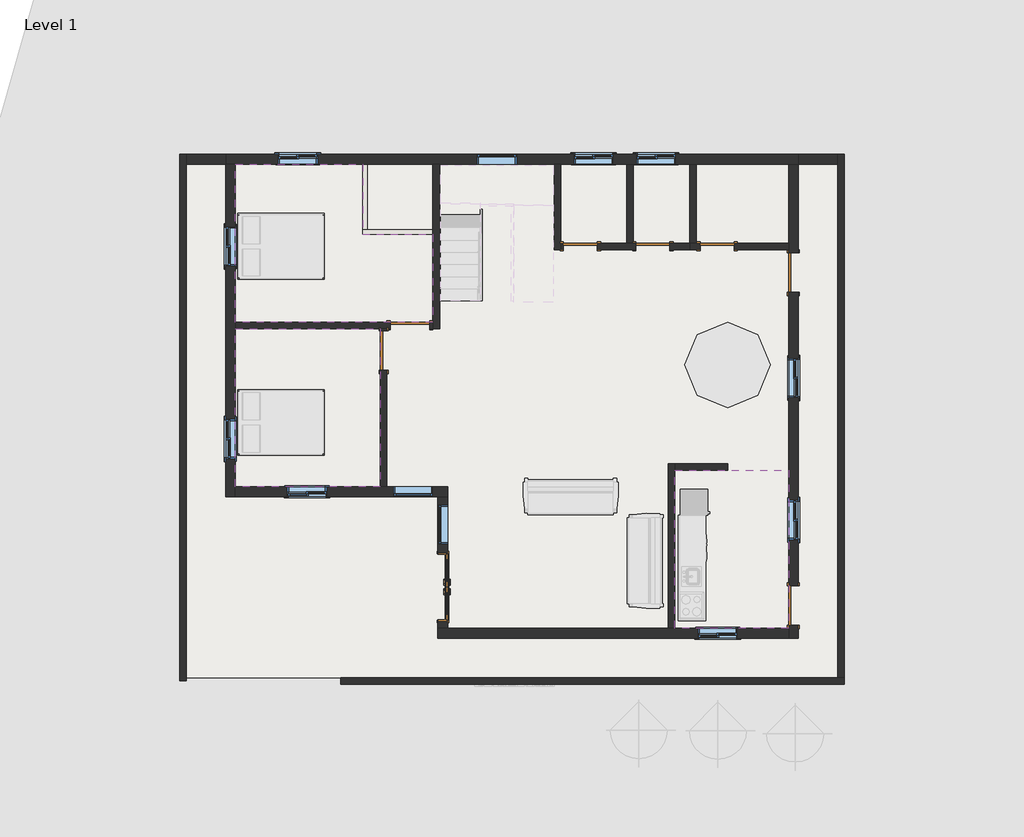
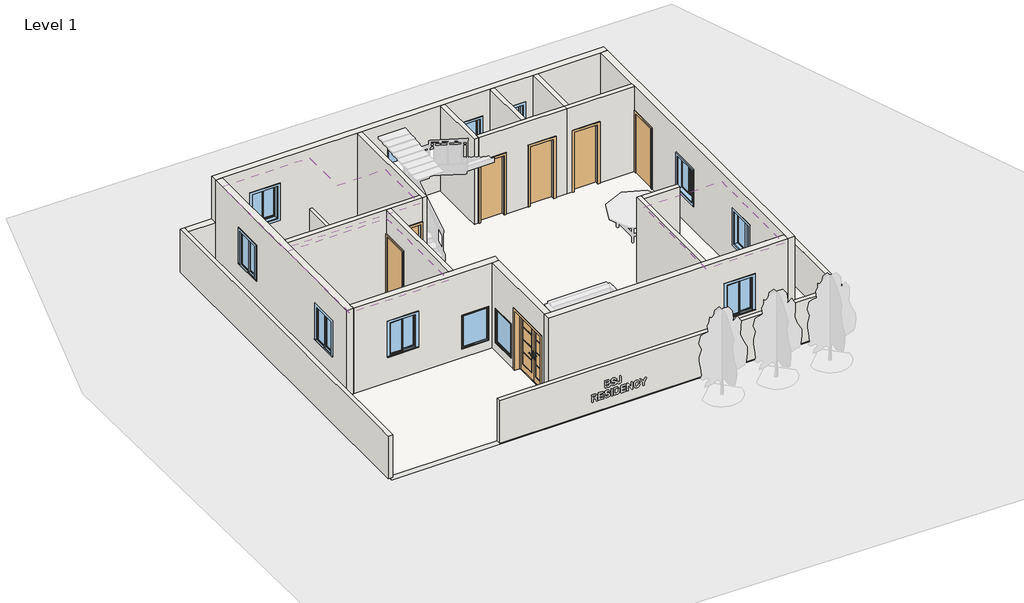
# One storey, part 1 of 2: 23 walls, 12 windows, 8 doors, 3 coverings, 1 slab.
"""IFC4 building model written with IfcOpenShell, lengths in millimetres."""

from ifc_helpers import new_model, si_unit, frame, origin, origin_with_axes, place, context, project, spatial, polyline, outline, extrude, faceted_brep, transform, mapped, element, save
from components import door_014e9f54, door_dc34e247, door_16372e1c, door_a90ba1ad, door_0ca8825f, window_c1f32544, window_26734613, window_e25db5b6

model = new_model("IFC4")

# Units and contexts
model_context = context("Model", 3, world=origin())
ifc_project = project(units=[si_unit("LENGTHUNIT", "METRE", prefix="MILLI")], contexts=[model_context])

# Site, building, storey
site = spatial("IfcSite", under=ifc_project)
building = spatial("IfcBuilding", under=site)
storey = spatial("IfcBuildingStorey", under=building, Name="Level 1", Elevation=0.0)

# Coverings
placement = place(None, origin())
element("IfcCovering", 1, ObjectType="2' x 4' ACT System", at=placement, inside=storey, context=model_context, shape_type="SweptSolid", body=[
    extrude(outline(polyline([(-8845.5867944, 6769.3230289), (-12198.3867944, 6769.3230289), (-12198.3867944, 10426.9230289), (-8845.5867944, 10426.9230289), (-8845.5867944, 6769.3230289)])), frame((0.0, 0.0, 2743.2), z_axis=(0.0, 0.0, 1.0), x_axis=(1.0, 0.0, 0.0)), (0.0, 0.0, 1.0), 57.15),
])
element("IfcCovering", 2, ObjectType="2' x 4' ACT System", at=placement, inside=storey, context=model_context, shape_type="SweptSolid", body=[
    extrude(outline(polyline([(-12198.3867944, 10579.3230289), (-12198.3867944, 14236.9230289), (-9251.9867944, 14236.9230289), (-9251.9867944, 12611.3230289), (-7626.3867944, 12611.3230289), (-7626.3867944, 10579.3230289), (-12198.3867944, 10579.3230289)])), frame((0.0, 0.0, 2743.2), z_axis=(0.0, 0.0, 1.0), x_axis=(1.0, 0.0, 0.0)), (0.0, 0.0, 1.0), 57.15),
])
element("IfcCovering", 3, ObjectType="2' x 4' ACT System", at=placement, inside=storey, context=model_context, shape_type="SweptSolid", body=[
    extrude(outline(polyline([(603.2132056, 7150.3230289), (603.2132056, 3492.7230289), (-2025.6867944, 3492.7230289), (-2025.6867944, 7150.3230289), (603.2132056, 7150.3230289)])), frame((0.0, 0.0, 2743.2), z_axis=(0.0, 0.0, 1.0), x_axis=(1.0, 0.0, 0.0)), (0.0, 0.0, 1.0), 57.15),
])

# Doors
door_shape = door_014e9f54(model_context)
element("IfcDoor", 4, ObjectType="Door-Exterior-Double-Full Glass-Wood_Clad : 60\" x 84\"", at=placement, inside=storey, context=model_context, shape_type="MappedRepresentation", body=[
    mapped(door_shape, transform((-7394.6117944, 4445.2230289, 0.0), x_axis=(0.0, -1.0, 0.0), y_axis=(1.0, 0.0, 0.0), z_axis=(0.0, 0.0, 1.0))),
])
door_2_shape = door_dc34e247(model_context)
element("IfcDoor", 5, ObjectType="Single-Flush : 2'7\"", at=placement, inside=storey, context=model_context, shape_type="MappedRepresentation", body=[
    mapped(door_2_shape, transform((-4212.7737939, 12331.9230289, 0.0), x_axis=(-1.0, 0.0, 0.0), y_axis=(0.0, -1.0, 0.0), z_axis=(0.0, 0.0, 1.0))),
])
element("IfcDoor", 6, ObjectType="Single-Flush : 2'7\"", at=placement, inside=storey, context=model_context, shape_type="MappedRepresentation", body=[
    mapped(door_2_shape, transform((-2536.3737939, 12331.9230289, 0.0), x_axis=(-1.0, 0.0, 0.0), y_axis=(0.0, -1.0, 0.0), z_axis=(0.0, 0.0, 1.0))),
])
element("IfcDoor", 7, ObjectType="Single-Flush : 2'7\"", at=placement, inside=storey, context=model_context, shape_type="MappedRepresentation", body=[
    mapped(door_2_shape, transform((-1047.7867944, 12331.9230289, 0.0), x_axis=(-1.0, 0.0, 0.0), y_axis=(0.0, -1.0, 0.0), z_axis=(0.0, 0.0, 1.0))),
])
door_3_shape = door_16372e1c(model_context)
element("IfcDoor", 8, ObjectType="Single-Flush : 36\" x 84\"", at=placement, inside=storey, context=model_context, shape_type="MappedRepresentation", body=[
    mapped(door_3_shape, transform((-8159.7867944, 10503.1230289, 0.0), x_axis=(1.0, 0.0, 0.0), y_axis=(0.0, 1.0, 0.0), z_axis=(0.0, 0.0, 1.0))),
])
element("IfcDoor", 9, ObjectType="Single-Flush : 36\" x 84\"", at=placement, inside=storey, context=model_context, shape_type="MappedRepresentation", body=[
    mapped(door_3_shape, transform((-8769.3867944, 9918.9230289, 0.0), x_axis=(0.0, 1.0, 0.0), y_axis=(-1.0, 0.0, 0.0), z_axis=(0.0, 0.0, 1.0))),
])
door_4_shape = door_a90ba1ad(model_context)
element("IfcDoor", 10, ObjectType="Single-Flush : 36\" x 84\"", at=placement, inside=storey, context=model_context, shape_type="MappedRepresentation", body=[
    mapped(door_4_shape, transform((717.5132056, 4013.4230289, 0.0), x_axis=(0.0, -1.0, 0.0), y_axis=(1.0, 0.0, 0.0), z_axis=(0.0, 0.0, 1.0))),
])
door_5_shape = door_0ca8825f(model_context)
element("IfcDoor", 11, ObjectType="Single-Flush : 36\" x 84\"", at=placement, inside=storey, context=model_context, shape_type="MappedRepresentation", body=[
    mapped(door_5_shape, transform((717.5132056, 11722.3230289, 0.0), x_axis=(0.0, 1.0, 0.0), y_axis=(-1.0, 0.0, 0.0), z_axis=(0.0, 0.0, 1.0))),
])

# Slab
element("IfcSlab", 12, ObjectType="6\"", at=placement, inside=storey, context=model_context, shape_type="SweptSolid", body=[
    extrude(outline(polyline([(1746.2132056, 14236.9230289), (1746.2132056, 2349.7230289), (-13341.3867944, 2349.7230289), (-13341.3867944, 14236.9230289), (1746.2132056, 14236.9230289)])), frame((0.0, 0.0, -152.4), z_axis=(0.0, 0.0, 1.0), x_axis=(1.0, 0.0, 0.0)), (0.0, 0.0, 1.0), 152.4),
])

# Walls
element("IfcWall", 13, ObjectType="4\"", at=placement, inside=storey, context=model_context, shape_type="Brep", body=[
    faceted_brep([(-7626.3867944, 12712.9230289, 0.0), (-9150.3867944, 12712.9230289, 0.0), (-9251.9867944, 12712.9230289, 0.0), (-9251.9867944, 12712.9230289, 914.4), (-9150.3867944, 12712.9230289, 914.4), (-7626.3867944, 12712.9230289, 914.4), (-7626.3867944, 12611.3230289, 0.0), (-7626.3867944, 12611.3230289, 914.4), (-9251.9867944, 12611.3230289, 914.4), (-9251.9867944, 12611.3230289, 0.0)], [[[0, 1, 2, 3, 4, 5]], [[6, 7, 8, 9]], [[2, 1, 0, 6, 9]], [[5, 4, 3, 8, 7]], [[0, 5, 7, 6]], [[3, 2, 9, 8]]]),
])
element("IfcWall", 14, ObjectType="4\"", at=placement, inside=storey, context=model_context, shape_type="SweptSolid", body=[
    extrude(outline(polyline([(-9150.3867944, 14236.9230289), (-9150.3867944, 12712.9230289), (-9251.9867944, 12712.9230289), (-9251.9867944, 14236.9230289), (-9150.3867944, 14236.9230289)])), origin_with_axes(), (0.0, 0.0, 1.0), 914.4),
])
element("IfcWall", 15, ObjectType="6\"", at=placement, inside=storey, context=model_context, shape_type="Brep", body=[
    faceted_brep([(-13341.3867944, 2273.5230289, 0.0), (-13341.3867944, 14236.9230289, 0.0), (-13341.3867944, 14465.5230289, 0.0), (-13341.3867944, 14465.5230289, 1524.0), (-13341.3867944, 14236.9230289, 1524.0), (-13341.3867944, 2273.5230289, 1524.0), (-13493.7867944, 2273.5230289, 0.0), (-13493.7867944, 2273.5230289, 1524.0), (-13493.7867944, 14465.5230289, 1524.0), (-13493.7867944, 14465.5230289, 0.0)], [[[0, 1, 2, 3, 4, 5]], [[6, 7, 8, 9]], [[2, 1, 0, 6, 9]], [[5, 4, 3, 8, 7]], [[0, 5, 7, 6]], [[3, 2, 9, 8]]]),
])
element("IfcWall", 16, ObjectType="6\"", at=placement, inside=storey, context=model_context, shape_type="Brep", body=[
    faceted_brep([(1898.6132056, 2349.7230289, 0.0), (1746.2132056, 2349.7230289, 0.0), (-9759.9867944, 2349.7230289, 0.0), (-9759.9867944, 2349.7230289, 1524.0), (1746.2132056, 2349.7230289, 1524.0), (1898.6132056, 2349.7230289, 1524.0), (1898.6132056, 2197.3230289, 0.0), (1898.6132056, 2197.3230289, 1524.0), (-9759.9867944, 2197.3230289, 1524.0), (-9759.9867944, 2197.3230289, 0.0)], [[[0, 1, 2, 3, 4, 5]], [[6, 7, 8, 9]], [[2, 1, 0, 6, 9]], [[3, 2, 9, 8]], [[5, 4, 3, 8, 7]], [[0, 5, 7, 6]]]),
])
element("IfcWall", 17, ObjectType="6\"", at=placement, inside=storey, context=model_context, shape_type="Brep", body=[
    faceted_brep([(1746.2132056, 14465.5230289, 0.0), (1746.2132056, 14236.9230289, 0.0), (1746.2132056, 2349.7230289, 0.0), (1746.2132056, 2349.7230289, 1524.0), (1746.2132056, 14236.9230289, 1524.0), (1746.2132056, 14465.5230289, 1524.0), (1898.6132056, 14465.5230289, 0.0), (1898.6132056, 14465.5230289, 1524.0), (1898.6132056, 2349.7230289, 1524.0), (1898.6132056, 2349.7230289, 0.0)], [[[0, 1, 2, 3, 4, 5]], [[6, 7, 8, 9]], [[2, 1, 0, 6, 9]], [[5, 4, 3, 8, 7]], [[3, 2, 9, 8]], [[0, 5, 7, 6]]]),
])
element("IfcWall", 18, ObjectType="6\"", at=placement, inside=storey, context=model_context, shape_type="Brep", body=[
    faceted_brep([(-7626.3867944, 14236.9230289, 0.0), (-7626.3867944, 12712.9230289, 0.0), (-7626.3867944, 12611.3230289, 0.0), (-7626.3867944, 10579.3230289, 0.0), (-7626.3867944, 10426.9230289, 0.0), (-7626.3867944, 10426.9230289, 3048.0), (-7626.3867944, 10579.3230289, 3048.0), (-7626.3867944, 14236.9230289, 3048.0), (-7473.9867944, 14236.9230289, 0.0), (-7473.9867944, 14236.9230289, 3048.0), (-7473.9867944, 10426.9230289, 3048.0), (-7473.9867944, 10426.9230289, 0.0)], [[[0, 1, 2, 3, 4, 5, 6, 7]], [[8, 9, 10, 11]], [[4, 3, 2, 1, 0, 8, 11]], [[7, 6, 5, 10, 9]], [[0, 7, 9, 8]], [[5, 4, 11, 10]]]),
])
element("IfcWall", 19, ObjectType="6\"", at=placement, inside=storey, context=model_context, shape_type="Brep", body=[
    faceted_brep([(-7626.3867944, 10579.3230289, 0.0), (-7702.5867944, 10579.3230289, 0.0), (-7702.5867944, 10579.3230289, 2133.6), (-8616.9867944, 10579.3230289, 2133.6), (-8616.9867944, 10579.3230289, 0.0), (-12198.3867944, 10579.3230289, 0.0), (-12198.3867944, 10579.3230289, 3048.0), (-7626.3867944, 10579.3230289, 3048.0), (-7702.5867944, 10426.9230289, 2133.6), (-7702.5867944, 10426.9230289, 0.0), (-7626.3867944, 10426.9230289, 0.0), (-7626.3867944, 10426.9230289, 3048.0), (-8693.1867944, 10426.9230289, 3048.0), (-8845.5867944, 10426.9230289, 3048.0), (-12198.3867944, 10426.9230289, 3048.0), (-12198.3867944, 10426.9230289, 0.0), (-8845.5867944, 10426.9230289, 0.0), (-8693.1867944, 10426.9230289, 0.0), (-8616.9867944, 10426.9230289, 0.0), (-8616.9867944, 10426.9230289, 2133.6)], [[[0, 1, 2, 3, 4, 5, 6, 7]], [[8, 9, 10, 11, 12, 13, 14, 15, 16, 17, 18, 19]], [[10, 9, 1, 0]], [[18, 17, 16, 15, 5, 4]], [[7, 6, 14, 13, 12, 11]], [[0, 7, 11, 10]], [[6, 5, 15, 14]], [[2, 1, 9, 8]], [[3, 2, 8, 19]], [[4, 3, 19, 18]]]),
])
element("IfcWall", 20, ObjectType="6\"", at=placement, inside=storey, context=model_context, shape_type="SweptSolid", body=[
    extrude(outline(polyline([(10426.9230289, 0.0), (10376.1230289, 0.0), (10376.1230289, 2133.6), (9461.7230289, 2133.6), (9461.7230289, 0.0), (6769.3230289, 0.0), (6769.3230289, 3048.0), (10426.9230289, 3048.0), (10426.9230289, 0.0)])), frame((-8845.5867944, 0.0, 0.0), z_axis=(1.0, 0.0, 0.0), x_axis=(0.0, 1.0, 0.0)), (0.0, 0.0, 1.0), 152.4),
])
element("IfcWall", 21, ObjectType="6\"", at=placement, inside=storey, context=model_context, shape_type="Brep", body=[
    faceted_brep([(-1441.4867944, 12408.1230289, 2133.6), (-1441.4867944, 12408.1230289, 0.0), (-1530.3867944, 12408.1230289, 0.0), (-1682.7867944, 12408.1230289, 0.0), (-1682.7867944, 12408.1230289, 3048.0), (-1530.3867944, 12408.1230289, 3048.0), (603.2132056, 12408.1230289, 3048.0), (603.2132056, 12408.1230289, 0.0), (-654.0867944, 12408.1230289, 0.0), (-654.0867944, 12408.1230289, 2133.6), (-1682.7867944, 12255.7230289, 0.0), (-1441.4867944, 12255.7230289, 0.0), (-1441.4867944, 12255.7230289, 2133.6), (-654.0867944, 12255.7230289, 2133.6), (-654.0867944, 12255.7230289, 0.0), (603.2132056, 12255.7230289, 0.0), (603.2132056, 12255.7230289, 3048.0), (-1682.7867944, 12255.7230289, 3048.0)], [[[0, 1, 2, 3, 4, 5, 6, 7, 8, 9]], [[10, 11, 12, 13, 14, 15, 16, 17]], [[8, 7, 15, 14]], [[3, 2, 1, 11, 10]], [[6, 5, 4, 17, 16]], [[7, 6, 16, 15]], [[4, 3, 10, 17]], [[12, 11, 1, 0]], [[13, 12, 0, 9]], [[14, 13, 9, 8]]]),
])
element("IfcWall", 22, ObjectType="6\"", at=placement, inside=storey, context=model_context, shape_type="SweptSolid", body=[
    extrude(outline(polyline([(-1530.3867944, 14236.9230289), (-1530.3867944, 12408.1230289), (-1682.7867944, 12408.1230289), (-1682.7867944, 14236.9230289), (-1530.3867944, 14236.9230289)])), origin_with_axes(), (0.0, 0.0, 1.0), 3048.0),
])
element("IfcWall", 23, ObjectType="6\"", at=placement, inside=storey, context=model_context, shape_type="Brep", body=[
    faceted_brep([(-4822.3737939, 14236.9230289, 0.0), (-4822.3737939, 12255.7230289, 0.0), (-4822.3737939, 12255.7230289, 3048.0), (-4822.3737939, 14236.9230289, 3048.0), (-4669.9737939, 14236.9230289, 0.0), (-4669.9737939, 14236.9230289, 3048.0), (-4669.9737939, 12408.1230289, 3048.0), (-4669.9737939, 12255.7230289, 3048.0), (-4669.9737939, 12255.7230289, 0.0), (-4669.9737939, 12408.1230289, 0.0)], [[[0, 1, 2, 3]], [[4, 5, 6, 7, 8, 9]], [[1, 0, 4, 9, 8]], [[3, 2, 7, 6, 5]], [[2, 1, 8, 7]], [[0, 3, 5, 4]]]),
])
element("IfcWall", 24, ObjectType="6\"", at=placement, inside=storey, context=model_context, shape_type="Brep", body=[
    faceted_brep([(-3819.0737939, 12255.7230289, 0.0), (-2930.0737939, 12255.7230289, 0.0), (-2930.0737939, 12255.7230289, 2133.6), (-2142.6737939, 12255.7230289, 2133.6), (-2142.6737939, 12255.7230289, 0.0), (-1682.7867944, 12255.7230289, 0.0), (-1682.7867944, 12255.7230289, 3048.0), (-4669.9737939, 12255.7230289, 3048.0), (-4669.9737939, 12255.7230289, 0.0), (-4606.4737939, 12255.7230289, 0.0), (-4606.4737939, 12255.7230289, 2133.6), (-3819.0737939, 12255.7230289, 2133.6), (-2930.0737939, 12408.1230289, 2133.6), (-2930.0737939, 12408.1230289, 0.0), (-2993.5737939, 12408.1230289, 0.0), (-3145.9737939, 12408.1230289, 0.0), (-3819.0737939, 12408.1230289, 0.0), (-3819.0737939, 12408.1230289, 2133.6), (-4606.4737939, 12408.1230289, 2133.6), (-4606.4737939, 12408.1230289, 0.0), (-4669.9737939, 12408.1230289, 0.0), (-4669.9737939, 12408.1230289, 3048.0), (-3145.9737939, 12408.1230289, 3048.0), (-2993.5737939, 12408.1230289, 3048.0), (-1682.7867944, 12408.1230289, 3048.0), (-1682.7867944, 12408.1230289, 0.0), (-2142.6737939, 12408.1230289, 0.0), (-2142.6737939, 12408.1230289, 2133.6)], [[[0, 1, 2, 3, 4, 5, 6, 7, 8, 9, 10, 11]], [[12, 13, 14, 15, 16, 17, 18, 19, 20, 21, 22, 23, 24, 25, 26, 27]], [[20, 19, 9, 8]], [[26, 25, 5, 4]], [[16, 15, 14, 13, 1, 0]], [[7, 6, 24, 23, 22, 21]], [[8, 7, 21, 20]], [[6, 5, 25, 24]], [[10, 9, 19, 18]], [[11, 10, 18, 17]], [[0, 11, 17, 16]], [[2, 1, 13, 12]], [[3, 2, 12, 27]], [[4, 3, 27, 26]]]),
])
element("IfcWall", 25, ObjectType="6\"", at=placement, inside=storey, context=model_context, shape_type="SweptSolid", body=[
    extrude(outline(polyline([(-2993.5737939, 14236.9230289), (-2993.5737939, 12408.1230289), (-3145.9737939, 12408.1230289), (-3145.9737939, 14236.9230289), (-2993.5737939, 14236.9230289)])), origin_with_axes(), (0.0, 0.0, 1.0), 3048.0),
])
element("IfcWall", 26, ObjectType="6\"", at=placement, inside=storey, context=model_context, shape_type="Brep", body=[
    faceted_brep([(-2025.6867944, 3492.7230289, 0.0), (-2025.6867944, 7150.3230289, 0.0), (-2025.6867944, 7302.7230289, 0.0), (-2025.6867944, 7302.7230289, 3048.0), (-2025.6867944, 7150.3230289, 3048.0), (-2025.6867944, 3492.7230289, 3048.0), (-2178.0867944, 3492.7230289, 0.0), (-2178.0867944, 3492.7230289, 3048.0), (-2178.0867944, 7302.7230289, 3048.0), (-2178.0867944, 7302.7230289, 0.0)], [[[0, 1, 2, 3, 4, 5]], [[6, 7, 8, 9]], [[2, 1, 0, 6, 9]], [[5, 4, 3, 8, 7]], [[0, 5, 7, 6]], [[3, 2, 9, 8]]]),
])
element("IfcWall", 27, ObjectType="6\"", at=placement, inside=storey, context=model_context, shape_type="SweptSolid", body=[
    extrude(outline(polyline([(-806.4867944, 7150.3230289), (-2025.6867944, 7150.3230289), (-2025.6867944, 7302.7230289), (-806.4867944, 7302.7230289), (-806.4867944, 7150.3230289)])), origin_with_axes(), (0.0, 0.0, 1.0), 3048.0),
])
element("IfcWall", 28, ObjectType="9\"", at=placement, inside=storey, context=model_context, shape_type="SweptSolid", body=[
    extrude(outline(polyline([(-12426.9867944, 14236.9230289), (-13341.3867944, 14236.9230289), (-13341.3867944, 14465.5230289), (-12426.9867944, 14465.5230289), (-12426.9867944, 14236.9230289)])), origin_with_axes(), (0.0, 0.0, 1.0), 1524.0),
])
element("IfcWall", 29, ObjectType="9\"", at=placement, inside=storey, context=model_context, shape_type="Brep", body=[
    faceted_brep([(-12426.9867944, 14236.9230289, 3048.0), (-12426.9867944, 14236.9230289, 0.0), (-12426.9867944, 6540.7230289, 0.0), (-12426.9867944, 6540.7230289, 3048.0), (-12426.9867944, 8331.4230289, 2133.6), (-12426.9867944, 7417.0230289, 2133.6), (-12426.9867944, 7417.0230289, 914.4), (-12426.9867944, 8331.4230289, 914.4), (-12426.9867944, 12789.1230289, 2133.6), (-12426.9867944, 11874.7230289, 2133.6), (-12426.9867944, 11874.7230289, 914.4), (-12426.9867944, 12789.1230289, 914.4), (-12198.3867944, 14236.9230289, 0.0), (-12198.3867944, 14236.9230289, 3048.0), (-12198.3867944, 10579.3230289, 3048.0), (-12198.3867944, 10426.9230289, 3048.0), (-12198.3867944, 6769.3230289, 3048.0), (-12198.3867944, 6540.7230289, 3048.0), (-12198.3867944, 6540.7230289, 0.0), (-12198.3867944, 6769.3230289, 0.0), (-12198.3867944, 10426.9230289, 0.0), (-12198.3867944, 10579.3230289, 0.0), (-12198.3867944, 8331.4230289, 2133.6), (-12198.3867944, 8331.4230289, 914.4), (-12198.3867944, 7417.0230289, 914.4), (-12198.3867944, 7417.0230289, 2133.6), (-12198.3867944, 12789.1230289, 2133.6), (-12198.3867944, 12789.1230289, 914.4), (-12198.3867944, 11874.7230289, 914.4), (-12198.3867944, 11874.7230289, 2133.6)], [[[0, 1, 2, 3], [4, 5, 6, 7], [8, 9, 10, 11]], [[12, 13, 14, 15, 16, 17, 18, 19, 20, 21], [22, 23, 24, 25], [26, 27, 28, 29]], [[2, 1, 12, 21, 20, 19, 18]], [[3, 2, 18, 17]], [[0, 3, 17, 16, 15, 14, 13]], [[23, 22, 4, 7]], [[24, 23, 7, 6]], [[25, 24, 6, 5]], [[22, 25, 5, 4]], [[27, 26, 8, 11]], [[28, 27, 11, 10]], [[29, 28, 10, 9]], [[26, 29, 9, 8]], [[0, 13, 12, 1]]]),
])
element("IfcWall", 30, ObjectType="9\"", at=placement, inside=storey, context=model_context, shape_type="Brep", body=[
    faceted_brep([(603.2132056, 14236.9230289, 0.0), (603.2132056, 12408.1230289, 0.0), (603.2132056, 12255.7230289, 0.0), (603.2132056, 12179.5230289, 0.0), (603.2132056, 12179.5230289, 2133.6), (603.2132056, 11265.1230289, 2133.6), (603.2132056, 11265.1230289, 0.0), (603.2132056, 4470.6230289, 0.0), (603.2132056, 4470.6230289, 2133.6), (603.2132056, 3556.2230289, 2133.6), (603.2132056, 3556.2230289, 0.0), (603.2132056, 3492.7230289, 0.0), (603.2132056, 3264.1230289, 0.0), (603.2132056, 3264.1230289, 3048.0), (603.2132056, 3492.7230289, 3048.0), (603.2132056, 12255.7230289, 3048.0), (603.2132056, 12408.1230289, 3048.0), (603.2132056, 14236.9230289, 3048.0), (603.2132056, 5537.4230289, 2133.6), (603.2132056, 5537.4230289, 914.4), (603.2132056, 6451.8230289, 914.4), (603.2132056, 6451.8230289, 2133.6), (603.2132056, 8826.7230289, 2133.6), (603.2132056, 8826.7230289, 914.4), (603.2132056, 9741.1230289, 914.4), (603.2132056, 9741.1230289, 2133.6), (831.8132056, 12179.5230289, 2133.6), (831.8132056, 12179.5230289, 0.0), (831.8132056, 14236.9230289, 0.0), (831.8132056, 14236.9230289, 3048.0), (831.8132056, 3264.1230289, 3048.0), (831.8132056, 3264.1230289, 0.0), (831.8132056, 3556.2230289, 0.0), (831.8132056, 3556.2230289, 2133.6), (831.8132056, 4470.6230289, 2133.6), (831.8132056, 4470.6230289, 0.0), (831.8132056, 11265.1230289, 0.0), (831.8132056, 11265.1230289, 2133.6), (831.8132056, 5537.4230289, 2133.6), (831.8132056, 6451.8230289, 2133.6), (831.8132056, 6451.8230289, 914.4), (831.8132056, 5537.4230289, 914.4), (831.8132056, 8826.7230289, 2133.6), (831.8132056, 9741.1230289, 2133.6), (831.8132056, 9741.1230289, 914.4), (831.8132056, 8826.7230289, 914.4)], [[[0, 1, 2, 3, 4, 5, 6, 7, 8, 9, 10, 11, 12, 13, 14, 15, 16, 17], [18, 19, 20, 21], [22, 23, 24, 25]], [[26, 27, 28, 29, 30, 31, 32, 33, 34, 35, 36, 37], [38, 39, 40, 41], [42, 43, 44, 45]], [[12, 11, 10, 32, 31]], [[36, 35, 7, 6]], [[28, 27, 3, 2, 1, 0]], [[17, 16, 15, 14, 13, 30, 29]], [[13, 12, 31, 30]], [[33, 32, 10, 9]], [[34, 33, 9, 8]], [[35, 34, 8, 7]], [[4, 3, 27, 26]], [[5, 4, 26, 37]], [[6, 5, 37, 36]], [[19, 18, 38, 41]], [[20, 19, 41, 40]], [[21, 20, 40, 39]], [[18, 21, 39, 38]], [[23, 22, 42, 45]], [[24, 23, 45, 44]], [[25, 24, 44, 43]], [[22, 25, 43, 42]], [[17, 29, 28, 0]]]),
])
element("IfcWall", 31, ObjectType="9\"", at=placement, inside=storey, context=model_context, shape_type="Brep", body=[
    faceted_brep([(603.2132056, 3492.7230289, 0.0), (-2025.6867944, 3492.7230289, 0.0), (-2178.0867944, 3492.7230289, 0.0), (-7283.4867944, 3492.7230289, 0.0), (-7512.0867944, 3492.7230289, 0.0), (-7512.0867944, 3492.7230289, 3048.0), (-7283.4867944, 3492.7230289, 3048.0), (-2178.0867944, 3492.7230289, 3048.0), (-2025.6867944, 3492.7230289, 3048.0), (603.2132056, 3492.7230289, 3048.0), (-1492.2867944, 3492.7230289, 2133.6), (-1492.2867944, 3492.7230289, 914.4), (-577.8867944, 3492.7230289, 914.4), (-577.8867944, 3492.7230289, 2133.6), (603.2132056, 3264.1230289, 0.0), (603.2132056, 3264.1230289, 3048.0), (-7512.0867944, 3264.1230289, 3048.0), (-7512.0867944, 3264.1230289, 0.0), (-1492.2867944, 3264.1230289, 2133.6), (-577.8867944, 3264.1230289, 2133.6), (-577.8867944, 3264.1230289, 914.4), (-1492.2867944, 3264.1230289, 914.4)], [[[0, 1, 2, 3, 4, 5, 6, 7, 8, 9], [10, 11, 12, 13]], [[14, 15, 16, 17], [18, 19, 20, 21]], [[4, 3, 2, 1, 0, 14, 17]], [[9, 8, 7, 6, 5, 16, 15]], [[0, 9, 15, 14]], [[5, 4, 17, 16]], [[11, 10, 18, 21]], [[12, 11, 21, 20]], [[13, 12, 20, 19]], [[10, 13, 19, 18]]]),
])
element("IfcWall", 32, ObjectType="9\"", at=placement, inside=storey, context=model_context, shape_type="Brep", body=[
    faceted_brep([(-12198.3867944, 6540.7230289, 0.0), (-7512.0867944, 6540.7230289, 0.0), (-7283.4867944, 6540.7230289, 0.0), (-7283.4867944, 6540.7230289, 3048.0), (-7512.0867944, 6540.7230289, 3048.0), (-12198.3867944, 6540.7230289, 3048.0), (-10998.2367944, 6540.7230289, 2133.6), (-10083.8367944, 6540.7230289, 2133.6), (-10083.8367944, 6540.7230289, 914.4), (-10998.2367944, 6540.7230289, 914.4), (-8540.7867944, 6540.7230289, 1524.0), (-7626.3867944, 6540.7230289, 1524.0), (-7626.3867944, 6540.7230289, 304.8), (-8540.7867944, 6540.7230289, 304.8), (-12198.3867944, 6769.3230289, 0.0), (-12198.3867944, 6769.3230289, 3048.0), (-8845.5867944, 6769.3230289, 3048.0), (-8693.1867944, 6769.3230289, 3048.0), (-7283.4867944, 6769.3230289, 3048.0), (-7283.4867944, 6769.3230289, 0.0), (-8693.1867944, 6769.3230289, 0.0), (-8845.5867944, 6769.3230289, 0.0), (-10998.2367944, 6769.3230289, 2133.6), (-10998.2367944, 6769.3230289, 914.4), (-10083.8367944, 6769.3230289, 914.4), (-10083.8367944, 6769.3230289, 2133.6), (-8540.7867944, 6769.3230289, 1524.0), (-8540.7867944, 6769.3230289, 304.8), (-7626.3867944, 6769.3230289, 304.8), (-7626.3867944, 6769.3230289, 1524.0)], [[[0, 1, 2, 3, 4, 5], [6, 7, 8, 9], [10, 11, 12, 13]], [[14, 15, 16, 17, 18, 19, 20, 21], [22, 23, 24, 25], [26, 27, 28, 29]], [[2, 1, 0, 14, 21, 20, 19]], [[5, 4, 3, 18, 17, 16, 15]], [[0, 5, 15, 14]], [[3, 2, 19, 18]], [[23, 22, 6, 9]], [[24, 23, 9, 8]], [[25, 24, 8, 7]], [[22, 25, 7, 6]], [[27, 26, 10, 13]], [[28, 27, 13, 12]], [[29, 28, 12, 11]], [[26, 29, 11, 10]]]),
])
element("IfcWall", 33, ObjectType="9\"", at=placement, inside=storey, context=model_context, shape_type="SweptSolid", body=[
    extrude(outline(polyline([(3492.7230289, 3048.0), (6540.7230289, 3048.0), (6540.7230289, 0.0), (5232.6230289, 0.0), (5232.6230289, 2159.0), (3657.8230289, 2159.0), (3657.8230289, 0.0), (3492.7230289, 0.0), (3492.7230289, 3048.0)]), holes=[polyline([(5435.8230289, 1524.0), (5435.8230289, 304.8), (6350.2230289, 304.8), (6350.2230289, 1524.0), (5435.8230289, 1524.0)])]), frame((-7512.0867944, 0.0, 0.0), z_axis=(1.0, 0.0, 0.0), x_axis=(0.0, 1.0, 0.0)), (0.0, 0.0, 1.0), 228.6),
])
element("IfcWall", 34, ObjectType="9\"", at=placement, inside=storey, context=model_context, shape_type="SweptSolid", body=[
    extrude(outline(polyline([(1746.2132056, 14236.9230289), (831.8132056, 14236.9230289), (831.8132056, 14465.5230289), (1746.2132056, 14465.5230289), (1746.2132056, 14236.9230289)])), origin_with_axes(), (0.0, 0.0, 1.0), 1524.0),
])
element("IfcWall", 35, ObjectType="9\"", at=placement, inside=storey, context=model_context, shape_type="Brep", body=[
    faceted_brep([(-12426.9867944, 14236.9230289, 0.0), (-12198.3867944, 14236.9230289, 0.0), (-9251.9867944, 14236.9230289, 0.0), (-9150.3867944, 14236.9230289, 0.0), (-7626.3867944, 14236.9230289, 0.0), (-7473.9867944, 14236.9230289, 0.0), (-4822.3737939, 14236.9230289, 0.0), (-4669.9737939, 14236.9230289, 0.0), (-3145.9737939, 14236.9230289, 0.0), (-2993.5737939, 14236.9230289, 0.0), (-1682.7867944, 14236.9230289, 0.0), (-1530.3867944, 14236.9230289, 0.0), (603.2132056, 14236.9230289, 0.0), (831.8132056, 14236.9230289, 0.0), (831.8132056, 14236.9230289, 1524.0), (831.8132056, 14236.9230289, 3048.0), (603.2132056, 14236.9230289, 3048.0), (-1530.3867944, 14236.9230289, 3048.0), (-1682.7867944, 14236.9230289, 3048.0), (-2993.5737939, 14236.9230289, 3048.0), (-3145.9737939, 14236.9230289, 3048.0), (-4669.9737939, 14236.9230289, 3048.0), (-4822.3737939, 14236.9230289, 3048.0), (-7473.9867944, 14236.9230289, 3048.0), (-7626.3867944, 14236.9230289, 3048.0), (-12198.3867944, 14236.9230289, 3048.0), (-12426.9867944, 14236.9230289, 3048.0), (-12426.9867944, 14236.9230289, 1524.0), (-10299.7367944, 14236.9230289, 2133.6), (-10299.7367944, 14236.9230289, 914.4), (-11214.1367944, 14236.9230289, 914.4), (-11214.1367944, 14236.9230289, 2133.6), (-2002.9737939, 14236.9230289, 2133.6), (-2002.9737939, 14236.9230289, 914.4), (-2917.3737939, 14236.9230289, 914.4), (-2917.3737939, 14236.9230289, 2133.6), (-3450.7737939, 14236.9230289, 2133.6), (-3450.7737939, 14236.9230289, 914.4), (-4365.1737939, 14236.9230289, 914.4), (-4365.1737939, 14236.9230289, 2133.6), (-5690.9802942, 14236.9230289, 2133.6), (-5690.9802942, 14236.9230289, 914.4), (-6605.3802942, 14236.9230289, 914.4), (-6605.3802942, 14236.9230289, 2133.6), (-12426.9867944, 14465.5230289, 0.0), (-12426.9867944, 14465.5230289, 1524.0), (-12426.9867944, 14465.5230289, 3048.0), (831.8132056, 14465.5230289, 3048.0), (831.8132056, 14465.5230289, 1524.0), (831.8132056, 14465.5230289, 0.0), (-10299.7367944, 14465.5230289, 2133.6), (-11214.1367944, 14465.5230289, 2133.6), (-11214.1367944, 14465.5230289, 914.4), (-10299.7367944, 14465.5230289, 914.4), (-2002.9737939, 14465.5230289, 2133.6), (-2917.3737939, 14465.5230289, 2133.6), (-2917.3737939, 14465.5230289, 914.4), (-2002.9737939, 14465.5230289, 914.4), (-3450.7737939, 14465.5230289, 2133.6), (-4365.1737939, 14465.5230289, 2133.6), (-4365.1737939, 14465.5230289, 914.4), (-3450.7737939, 14465.5230289, 914.4), (-5690.9802942, 14465.5230289, 2133.6), (-6605.3802942, 14465.5230289, 2133.6), (-6605.3802942, 14465.5230289, 914.4), (-5690.9802942, 14465.5230289, 914.4)], [[[0, 1, 2, 3, 4, 5, 6, 7, 8, 9, 10, 11, 12, 13, 14, 15, 16, 17, 18, 19, 20, 21, 22, 23, 24, 25, 26, 27], [28, 29, 30, 31], [32, 33, 34, 35], [36, 37, 38, 39], [40, 41, 42, 43]], [[44, 45, 46, 47, 48, 49], [50, 51, 52, 53], [54, 55, 56, 57], [58, 59, 60, 61], [62, 63, 64, 65]], [[13, 12, 11, 10, 9, 8, 7, 6, 5, 4, 3, 2, 1, 0, 44, 49]], [[15, 14, 13, 49, 48, 47]], [[26, 25, 24, 23, 22, 21, 20, 19, 18, 17, 16, 15, 47, 46]], [[0, 27, 26, 46, 45, 44]], [[28, 31, 51, 50]], [[31, 30, 52, 51]], [[30, 29, 53, 52]], [[29, 28, 50, 53]], [[32, 35, 55, 54]], [[35, 34, 56, 55]], [[34, 33, 57, 56]], [[33, 32, 54, 57]], [[36, 39, 59, 58]], [[39, 38, 60, 59]], [[38, 37, 61, 60]], [[37, 36, 58, 61]], [[40, 43, 63, 62]], [[43, 42, 64, 63]], [[42, 41, 65, 64]], [[41, 40, 62, 65]]]),
])

# Windows
window_shape = window_c1f32544(model_context)
element("IfcWindow", 36, ObjectType="Fixed : 36\" x 48\"", at=placement, inside=storey, context=model_context, shape_type="MappedRepresentation", body=[
    mapped(window_shape, transform((-6110.0802942, 14351.2230289, 0.0), x_axis=(1.0, 0.0, 0.0), y_axis=(0.0, 1.0, 0.0), z_axis=(0.0, 0.0, 1.0))),
])
element("IfcWindow", 37, ObjectType="Fixed : 36\" x 48\"", at=placement, inside=storey, context=model_context, shape_type="MappedRepresentation", body=[
    mapped(window_shape, transform((-8121.6867944, 6655.0230289, -609.6), x_axis=(-1.0, 0.0, 0.0), y_axis=(0.0, -1.0, 0.0), z_axis=(0.0, 0.0, 1.0))),
])
window_2_shape = window_26734613(model_context)
element("IfcWindow", 38, ObjectType="Fixed : 36\" x 48\"", at=placement, inside=storey, context=model_context, shape_type="MappedRepresentation", body=[
    mapped(window_2_shape, transform((-7397.7867944, 5854.9230289, -609.6), x_axis=(0.0, -1.0, 0.0), y_axis=(1.0, 0.0, 0.0), z_axis=(0.0, 0.0, 1.0))),
])
window_3_shape = window_e25db5b6(model_context)
element("IfcWindow", 39, ObjectType="Slider with Trim : 36\" x 48\"", at=placement, inside=storey, context=model_context, shape_type="MappedRepresentation", body=[
    mapped(window_3_shape, transform((-12312.6867944, 7874.2230289, 0.0), x_axis=(0.0, 1.0, 0.0), y_axis=(-1.0, 0.0, 0.0), z_axis=(0.0, 0.0, 1.0))),
])
element("IfcWindow", 40, ObjectType="Slider with Trim : 36\" x 48\"", at=placement, inside=storey, context=model_context, shape_type="MappedRepresentation", body=[
    mapped(window_3_shape, transform((-12312.6867944, 12331.9230289, 0.0), x_axis=(0.0, 1.0, 0.0), y_axis=(-1.0, 0.0, 0.0), z_axis=(0.0, 0.0, 1.0))),
])
element("IfcWindow", 41, ObjectType="Slider with Trim : 36\" x 48\"", at=placement, inside=storey, context=model_context, shape_type="MappedRepresentation", body=[
    mapped(window_3_shape, transform((-10756.9367944, 14351.2230289, 0.0), x_axis=(1.0, 0.0, 0.0), y_axis=(0.0, 1.0, 0.0), z_axis=(0.0, 0.0, 1.0))),
])
element("IfcWindow", 42, ObjectType="Slider with Trim : 36\" x 48\"", at=placement, inside=storey, context=model_context, shape_type="MappedRepresentation", body=[
    mapped(window_3_shape, transform((-10541.0367944, 6655.0230289, 0.0), x_axis=(-1.0, 0.0, 0.0), y_axis=(0.0, -1.0, 0.0), z_axis=(0.0, 0.0, 1.0))),
])
element("IfcWindow", 43, ObjectType="Slider with Trim : 36\" x 48\"", at=placement, inside=storey, context=model_context, shape_type="MappedRepresentation", body=[
    mapped(window_3_shape, transform((-1035.0867944, 3378.4230289, 0.0), x_axis=(-1.0, 0.0, 0.0), y_axis=(0.0, -1.0, 0.0), z_axis=(0.0, 0.0, 1.0))),
])
element("IfcWindow", 44, ObjectType="Slider with Trim : 36\" x 48\"", at=placement, inside=storey, context=model_context, shape_type="MappedRepresentation", body=[
    mapped(window_3_shape, transform((717.5132056, 5994.6230289, 0.0), x_axis=(0.0, -1.0, 0.0), y_axis=(1.0, 0.0, 0.0), z_axis=(0.0, 0.0, 1.0))),
])
element("IfcWindow", 45, ObjectType="Slider with Trim : 36\" x 48\"", at=placement, inside=storey, context=model_context, shape_type="MappedRepresentation", body=[
    mapped(window_3_shape, transform((717.5132056, 9283.9230289, 0.0), x_axis=(0.0, -1.0, 0.0), y_axis=(1.0, 0.0, 0.0), z_axis=(0.0, 0.0, 1.0))),
])
element("IfcWindow", 46, ObjectType="Slider with Trim : 36\" x 48\"", at=placement, inside=storey, context=model_context, shape_type="MappedRepresentation", body=[
    mapped(window_3_shape, transform((-2460.1737939, 14351.2230289, 0.0), x_axis=(1.0, 0.0, 0.0), y_axis=(0.0, 1.0, 0.0), z_axis=(0.0, 0.0, 1.0))),
])
element("IfcWindow", 47, ObjectType="Slider with Trim : 36\" x 48\"", at=placement, inside=storey, context=model_context, shape_type="MappedRepresentation", body=[
    mapped(window_3_shape, transform((-3907.9737939, 14351.2230289, 0.0), x_axis=(1.0, 0.0, 0.0), y_axis=(0.0, 1.0, 0.0), z_axis=(0.0, 0.0, 1.0))),
])

save(model, "model.ifc")

# Revit data of these elements
# Type "2' x 4' ACT System"
#   Assembly Code = "C3030210"
#   built-in parameter 1002203 = 1 (stored number, unit not read)
#   built-in parameter 1002202 = 1 (stored number, unit not read)
#   Layers, outside or top first: 0' - 1 5/8" "Default" (function 1); 0' - 0 5/8" "Softwood, Lumber" (function 5)
# Type "Door-Exterior-Double-Full Glass-Wood_Clad : 60\" x 84\""
#   Type Mark = "9"
#   Assembly Code = "B2030100"
#   Analytic Construction = "French door, wood frame with double glass"
#   Top Rail = 0' - 4 11/16"
#   Threshold Offset [instance default] = 0' - 0 1/2"
#   Thickness = 0' - 1 3/8"
#   Thermal Resistance (R) = 1.9158 (h·ft²·°F)/BTU
#   Swing Angle [instance default] = 90.00°
#   Stiles = 0' - 4 3/4"
#   Rough Width = 5' - 2"
#   Rough Height = 7' - 1"
#   Panel Width = 2' - 6"
#   Door Offset [instance default] = 0' - 0"
#   Height = 7' - 0"
#   Width = 5' - 0"
#   Heat Transfer Coefficient (U) = 0.5220 BTU/(h·ft²·°F)
#   Bottom Rail = 0' - 9 1/8"
#   Exterior Trim [instance default] = yes
#   Threshold [instance default] = yes
#   Show Grill [instance default] = yes
#   Function = 1
#   Trim Material = Cherry
#   Threshold Material = Cherry
#   Panel Material = Cherry
#   Glazing = Glass
#   Frame Material = Cherry
#   Door Handle Material = Aluminum
#   Visual Light Transmittance = 0
#   Solar Heat Gain Coefficient = 0
#   Wall Closure = (empty or 0)
#   Construction Type = (empty or 0)
# Type "Single-Flush : 2'7\""
#   Type Mark = "8"
#   Construction Type Id = "MDOOR"
#   Assembly Code = "C1020"
#   Analytic Construction = "Metal"
#   Thickness = 0' - 2"
#   Heat Transfer Coefficient (U) = 0.651978 BTU/(h·ft²·°F)
#   Height = 7' - 0"
#   Trim Projection Ext = 0' - 1"
#   Trim Projection Int = 0' - 1"
#   Trim Width = 0' - 3"
#   Width = 2' - 7"
#   Define Thermal Properties by = 1
#   Door Material = Door - Panel
#   Frame Material = Door - Frame
#   Visual Light Transmittance = 0
#   Solar Heat Gain Coefficient = 0
#   Function = (empty or 0)
#   Wall Closure = (empty or 0)
# Type "Single-Flush : 36\" x 84\""
#   Type Mark = "1"
#   Construction Type Id = "MDOOR"
#   Assembly Code = "C1020"
#   Analytic Construction = "Metal"
#   Thickness = 0' - 2"
#   Heat Transfer Coefficient (U) = 0.651978 BTU/(h·ft²·°F)
#   Height = 7' - 0"
#   Trim Projection Ext = 0' - 1"
#   Trim Projection Int = 0' - 1"
#   Trim Width = 0' - 3"
#   Width = 3' - 0"
#   Define Thermal Properties by = 1
#   Door Material = Door - Panel
#   Frame Material = Door - Frame
#   Visual Light Transmittance = 0
#   Solar Heat Gain Coefficient = 0
#   Function = (empty or 0)
#   Wall Closure = (empty or 0)
# Type "6\""
#   Assembly Code = "B1010"
#   Function = 0
#   Layers, outside or top first: 0' - 6" "flooring" (function 1)
# Type "4\""
#   Assembly Code = "B2010"
#   Layers, outside or top first: 0' - 4" "EXT WALL" (function 1)
# Type "6\""
#   Assembly Code = "B2010"
#   Layers, outside or top first: 0' - 6" "INT WALL" (function 1)
# Type "9\""
#   Assembly Code = "B2010"
#   Layers, outside or top first: 0' - 9" "EXT WALL" (function 1)
# Type "Fixed : 36\" x 48\""
#   Type Mark = "9"
#   Construction Type Id = "GSP4R"
#   Assembly Code = "B2020100"
#   Analytic Construction = "1/8 in Pilkington single glazing"
#   Visual Light Transmittance = 0.9
#   Solar Heat Gain Coefficient = 0.78
#   Heat Transfer Coefficient (U) = 0.6496 BTU/(h·ft²·°F)
#   Height = 4' - 0"
#   Default Sill Height = 3' - 0"
#   Width = 3' - 0"
#   Window Inset = 0' - 0 3/4"
#   Define Thermal Properties by = 1
#   Wall Closure = 3
#   Glass Pane Material = Glass
#   Sash Material = Sash
# Type "Slider with Trim : 36\" x 48\""
#   Type Mark = "10"
#   Construction Type Id = "GSP4R"
#   Assembly Code = "B2020100"
#   Analytic Construction = "1/8 in Pilkington single glazing"
#   Visual Light Transmittance = 0.9
#   Solar Heat Gain Coefficient = 0.78
#   Heat Transfer Coefficient (U) = 0.6496 BTU/(h·ft²·°F)
#   Height = 4' - 0"
#   Default Sill Height = 3' - 0"
#   Trim Projection - Ext. = 0' - 0 3/4"
#   Trim Projection - Int. = 0' - 0 3/4"
#   Trim Width - Exterior = 0' - 3 1/2"
#   Trim Width - Interior = 0' - 3 1/2"
#   Width = 3' - 0"
#   Window Inset = 0' - 0 3/4"
#   Define Thermal Properties by = 1
#   Glass Pane Material = Glass
#   Sash Material = Sash
#   Trim Exterior Material = Trim
#   Trim Interior Material = Trim
#   Wall Closure = (empty or 0)
# Elements 1, 2, 3 (IfcCovering, "2' x 4' ACT System")
#   Height Offset From Level = 9' - 0"
#   Phase Created = New Construction
#   Materials on its faces: "Softwood, Lumber", "Default"
# Element 4 (IfcDoor, "Door-Exterior-Double-Full Glass-Wood_Clad : 60\" x 84\"")
#   Threshold Offset = 0' - 0 1/2"
#   Swing Angle = 90.00°
#   Door Offset = 0' - 0"
#   Threshold = yes
#   Show Grill = yes
#   Exterior Trim = yes
#   Phase Created = New Construction
#   Materials on its faces: "Cherry", "Aluminum", "Glass"
# Elements 5, 6, 7 (IfcDoor, "Single-Flush : 2'7\"")
#   Phase Created = New Construction
#   Materials on its faces: "Door - Frame", "Door - Panel"
# Elements 8, 9, 10, 11 (IfcDoor, "Single-Flush : 36\" x 84\"")
#   Phase Created = New Construction
#   Materials on its faces: "Door - Frame", "Door - Panel"
# Element 12 (IfcSlab, "6\"")
#   Height Offset From Level = 0' - 0"
#   Phase Created = New Construction
#   Materials on its faces: "flooring"
# Elements 13, 14 (IfcWall, "4\"")
#   Top Offset = 0' - 0"
#   Base Offset = 0' - 0"
#   Unconnected Height = 3' - 0"
#   wall height = 3' - 0"
#   Phase Created = New Construction
#   Base Constraint = Level 1
#   Materials on its faces: "EXT WALL"
# Elements 15, 17 (IfcWall, "6\"")
#   Top Offset = 0' - 0"
#   Base Offset = 0' - 0"
#   Unconnected Height = 5' - 0"
#   wall height = 5' - 0"
#   Phase Created = New Construction
#   Base Constraint = Level 1
#   Materials on its faces: "INT WALL", "EXT WALL"
# Element 16 (IfcWall, "6\"")
#   Top Offset = 0' - 0"
#   Base Offset = 0' - 0"
#   Unconnected Height = 5' - 0"
#   wall height = 5' - 0"
#   Phase Created = New Construction
#   Base Constraint = Level 1
#   Materials on its faces: "INT WALL"
# Elements 18, 19, 20, 21, 22, 23, 24, 25, 26, 27 (IfcWall, "6\"")
#   Top Offset = 0' - 0"
#   Base Offset = 0' - 0"
#   Unconnected Height = 10' - 0"
#   wall height = 10' - 0"
#   Phase Created = New Construction
#   Base Constraint = Level 1
#   Materials on its faces: "INT WALL"
# Elements 28, 34 (IfcWall, "9\"")
#   Top Offset = 0' - 0"
#   Base Offset = 0' - 0"
#   Unconnected Height = 5' - 0"
#   wall height = 5' - 0"
#   Phase Created = New Construction
#   Base Constraint = Level 1
#   Materials on its faces: "EXT WALL"
# Elements 29, 30, 31, 32, 33, 35 (IfcWall, "9\"")
#   Top Offset = 0' - 0"
#   Base Offset = 0' - 0"
#   Unconnected Height = 10' - 0"
#   wall height = 10' - 0"
#   Phase Created = New Construction
#   Base Constraint = Level 1
#   Materials on its faces: "EXT WALL"
# Element 36 (IfcWindow, "Fixed : 36\" x 48\"")
#   Mark = "11"
#   Phase Created = New Construction
#   Materials on its faces: "Sash", "Glass"
# Element 37 (IfcWindow, "Fixed : 36\" x 48\"")
#   Mark = "12"
#   Phase Created = New Construction
#   Materials on its faces: "Sash", "Glass"
# Element 38 (IfcWindow, "Fixed : 36\" x 48\"")
#   Mark = "13"
#   Phase Created = New Construction
#   Materials on its faces: "Sash", "Glass"
# Element 39 (IfcWindow, "Slider with Trim : 36\" x 48\"")
#   Mark = "1"
#   Phase Created = New Construction
#   Materials on its faces: "Sash", "Trim", "Glass"
# Element 40 (IfcWindow, "Slider with Trim : 36\" x 48\"")
#   Mark = "2"
#   Phase Created = New Construction
#   Materials on its faces: "Sash", "Trim", "Glass"
# Element 41 (IfcWindow, "Slider with Trim : 36\" x 48\"")
#   Mark = "3"
#   Phase Created = New Construction
#   Materials on its faces: "Sash", "Trim", "Glass"
# Element 42 (IfcWindow, "Slider with Trim : 36\" x 48\"")
#   Mark = "4"
#   Phase Created = New Construction
#   Materials on its faces: "Sash", "Trim", "Glass"
# Element 43 (IfcWindow, "Slider with Trim : 36\" x 48\"")
#   Mark = "5"
#   Phase Created = New Construction
#   Materials on its faces: "Sash", "Trim", "Glass"
# Element 44 (IfcWindow, "Slider with Trim : 36\" x 48\"")
#   Mark = "6"
#   Phase Created = New Construction
#   Materials on its faces: "Sash", "Trim", "Glass"
# Element 45 (IfcWindow, "Slider with Trim : 36\" x 48\"")
#   Mark = "7"
#   Phase Created = New Construction
#   Materials on its faces: "Sash", "Trim", "Glass"
# Element 46 (IfcWindow, "Slider with Trim : 36\" x 48\"")
#   Mark = "8"
#   Phase Created = New Construction
#   Materials on its faces: "Sash", "Trim", "Glass"
# Element 47 (IfcWindow, "Slider with Trim : 36\" x 48\"")
#   Mark = "9"
#   Phase Created = New Construction
#   Materials on its faces: "Sash", "Trim", "Glass"
# Materials
#   "Default": colour RGB 127 127 127, transparency 0
#   "Softwood, Lumber": class "Wood", colour RGB 144 112 60, transparency 0, Description = "Pinus Echinata", Cost = 0
#   "Cherry": class "Wood", colour RGB 226 177 128, transparency 0, Description = "Prunus Serotina", Cost = 0
#   "Glass": class "Glass", colour RGB 0 128 192, transparency 0.75, Description = "Soda Lime Glass", Cost = 0
#   "Aluminum": class "Metal", colour RGB 247 247 247, transparency 0, Description = "Aluminum 6061", Cost = 0
#   "Door - Panel": class "Wood", colour RGB 210 159 95, transparency 0
#   "Door - Frame": colour RGB 118 70 51, transparency 0
#   "flooring": class "Generic", colour RGB 120 120 120, transparency 0, Cost = 0
#   "EXT WALL": class "Generic", colour RGB 159 125 47, transparency 0, Cost = 0
#   "INT WALL": class "Generic", colour RGB 187 179 160, transparency 0, Cost = 0
#   "Sash": class "Wood", colour RGB 224 178 126, transparency 0
#   "Trim": class "Wood", colour RGB 224 178 126, transparency 0
